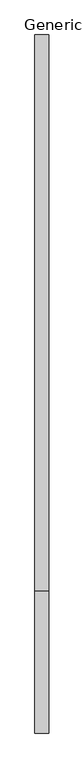
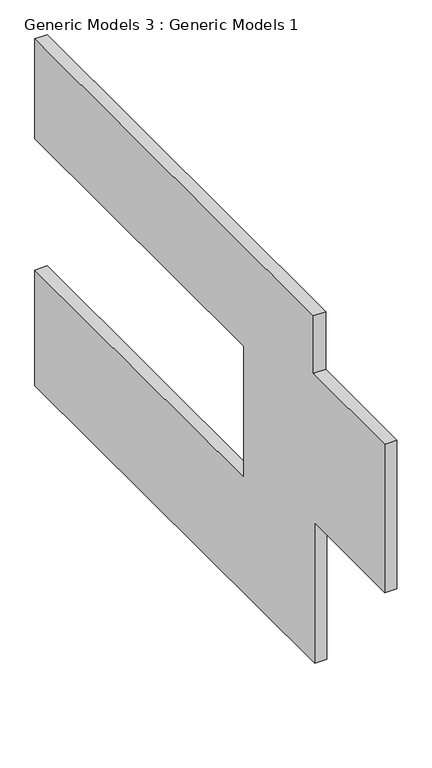
"""IFC4 building model written with IfcOpenShell, lengths in millimetres: proxy geometry, Generic Models 3 : Generic Models 1."""

from ifc_helpers import new_model, si_unit, frame, origin, place, context, project, spatial, polyline, outline, extrude, source, transform, mapped, element, save


def generic_models_3_generic_models_1_fe68d0d7(model_context):
    return source(origin(), model_context, "Body", "SweptSolid", [
        extrude(outline(polyline([(-3946.8023495, -1492.25), (-3946.8023495, 2214.7139463), (-6979.1363705, 2214.7139463), (-6979.1363705, 6127.75), (-3899.3863708, 6127.75), (-3899.3863708, 7651.75), (8140.2136292, 7651.75), (8140.2136292, 5015.8429185), (-883.1363705, 5015.8429185), (-883.1363705, 1555.75), (8140.2136292, 1555.75), (8140.2136292, -1492.25), (-3946.8023495, -1492.25)])), frame((13902.5156363, 0.0, 0.0), z_axis=(1.0, 0.0, 0.0), x_axis=(0.0, 1.0, 0.0)), (0.0, 0.0, 1.0), 304.8),
    ])


if __name__ == "__main__":
    model = new_model("IFC4")
    model_context = context("Model", 3, world=origin())
    ifc_project = project(units=[si_unit("LENGTHUNIT", "METRE", prefix="MILLI")], contexts=[model_context])
    site = spatial("IfcSite", under=ifc_project)
    building = spatial("IfcBuilding", under=site)
    placement = place(None, origin())
    generic_models_3_generic_models_1_shape = generic_models_3_generic_models_1_fe68d0d7(model_context)
    element("IfcBuildingElementProxy", 1, Name="Generic Models 3 : Generic Models 1", ObjectType="Generic Models 3 : Generic Models 1", at=placement, inside=building, context=model_context, shape_type="MappedRepresentation", body=[
        mapped(generic_models_3_generic_models_1_shape, transform((0.0, 0.0, 0.0), x_axis=(1.0, 0.0, 0.0), y_axis=(0.0, 1.0, 0.0), z_axis=(0.0, 0.0, 1.0))),
    ])
    save(model, "model.ifc")
